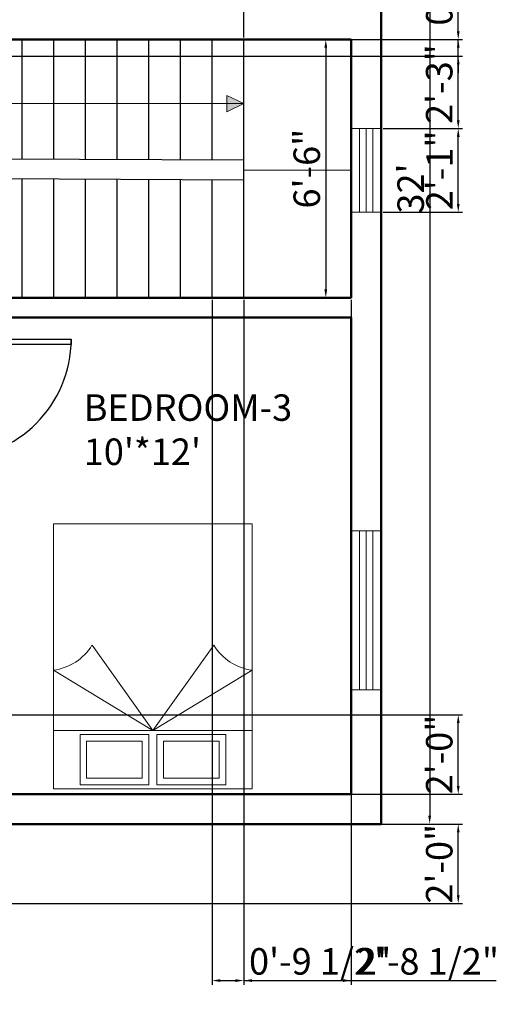
# Model space of a CAD drawing. Units: inches. Extents: x 2528 to 2954, y 1660 to 2209.
# Tile 3 of 4: x 2810 to 2954, y 1660 to 1957. Entities that reach past the tile are written whole.
import ezdxf

# ---------------------------------------------------------------- set-up
doc = ezdxf.new("R2010")
doc.units = ezdxf.units.IN
for name, color, linetype, lineweight in [('A-ANNO-DIMS', 5, 'Continuous', 18), ('A-ANNO-SYMB', 5, 'Continuous', 18), ('A-AREA-IDEN', 5, 'Continuous', 25), ('DOOR', 3, 'Continuous', 25), ('FURNITURE', 6, 'Continuous', 18), ('STEPS', 30, 'Continuous', 25), ('WALL', 1, 'Continuous', 50), ('WINDOW', 4, 'Continuous', 18)]:
    doc.layers.add(name, color=color, linetype=linetype, lineweight=lineweight)
doc.styles.get("Standard").update_dxf_attribs({"font": 'arial.ttf'})
doc.dimstyles.new('ISO-25', dxfattribs={"dimtxt": 8, "dimasz": 2.5, "dimexe": 1.25, "dimexo": 0.625, "dimtad": 1, "dimlunit": 3, "dimtxsty": 'Standard', "dimcen": 2.5, "dimadec": 0, "dimazin": 0, "dimtfac": 1, "dimtmove": 0, "dimatfit": 3, "dimfxl": 1, "dimarcsym": 0})

# ---------------------------------------------------------------- blocks, each defined once
blk = doc.blocks.new('*U2')
for p, q in [((0, 0), (0, -6)), ((40, 0), (40, -6))]:
    blk.add_line(p, q)
blk.add_lwpolyline([(0, 0), (0, 40), (1.75, 40), (1.75, 0)], close=True)
blk.add_arc((0, 0), 40, 0, 90)
blk = doc.blocks.new('*D12')
at = {"layer": 'A-ANNO-DIMS', "color": 0, "lineweight": -2, "transparency": 16777216}
for p, q in [((2919.54, 2098.39), (2934.84, 2098.39)), ((2933.59, 2095.89), (2933.59, 1716.89)), ((2919.54, 1714.39), (2934.84, 1714.39))]:
    blk.add_line(p, q, dxfattribs=at)
at = {"layer": 'A-ANNO-DIMS', "color": 0, "transparency": 16777216}
for points in [[(2933.17, 2095.89), (2934.01, 2095.89), (2933.59, 2098.39)], [(2933.17, 1716.89), (2934.01, 1716.89), (2933.59, 1714.39)]]:
    blk.add_solid(points, dxfattribs=at)
at = {"layer": 'Defpoints', "color": 0, "transparency": 16777216}
for p in [(2918.92, 2098.39), (2918.92, 1714.39), (2933.59, 1714.39)]:
    blk.add_point(p, dxfattribs=at)
at = {"layer": 'A-ANNO-DIMS', "color": 0, "transparency": 16777216, "insert": (2928.88, 1906.39), "char_height": 8, "attachment_point": 5, "rotation": 90}
blk.add_mtext("32'", dxfattribs=at)
blk = doc.blocks.new('*D13')
at = {"layer": 'A-ANNO-DIMS', "color": 0, "lineweight": -2, "transparency": 16777216}
for p, q in [((2878.05, 1951.39), (2903.46, 1951.39)), ((2902.21, 1948.89), (2902.21, 1875.89)), ((2878.05, 1873.39), (2903.46, 1873.39))]:
    blk.add_line(p, q, dxfattribs=at)
at = {"layer": 'A-ANNO-DIMS', "color": 0, "transparency": 16777216}
for points in [[(2901.79, 1948.89), (2902.63, 1948.89), (2902.21, 1951.39)], [(2901.79, 1875.89), (2902.63, 1875.89), (2902.21, 1873.39)]]:
    blk.add_solid(points, dxfattribs=at)
at = {"layer": 'Defpoints', "color": 0, "transparency": 16777216}
for p in [(2877.42, 1951.39), (2877.42, 1873.39), (2902.21, 1873.39)]:
    blk.add_point(p, dxfattribs=at)
at = {"layer": 'A-ANNO-DIMS', "color": 0, "transparency": 16777216, "insert": (2897.5, 1912.39), "char_height": 8, "attachment_point": 5, "rotation": 90}
blk.add_mtext('6\'-6"', dxfattribs=at)
blk = doc.blocks.new('BED-QUEEN-60X80')
for p, q in [((0, 0), (0, 80)), ((0, 80), (60, 80)), ((8, 78.8), (28.8, 78.8)), ((8, 65.6), (8, 78.8)), ((28.8, 78.8), (28.8, 63.6)), ((31.2, 78.8), (52, 78.8)), ((31.2, 65.6), (31.2, 78.8)), ((52, 78.8), (52, 63.6)), ((60, 80), (60, 0)), ((10, 76.8), (26.8, 76.8)), ((10, 65.6), (10, 76.8)), ((26.8, 76.8), (26.8, 65.6)), ((33.2, 65.6), (33.2, 76.8)), ((33.2, 76.8), (50, 76.8)), ((50, 76.8), (50, 65.6)), ((8, 63.6), (8, 65.6)), ((26.8, 65.6), (10, 65.6)), ((31.2, 63.6), (31.2, 65.6)), ((50, 65.6), (33.2, 65.6)), ((28.8, 63.6), (8, 63.6)), ((52, 63.6), (31.2, 63.6)), ((60, 62.4), (0, 62.4)), ((30, 62.4), (0, 44.18)), ((11.62, 36.62), (30, 62.4)), ((30, 62.4), (60, 44.18)), ((48.38, 36.62), (30, 62.4)), ((52, 62.4), (31.2, 62.4)), ((60, 0), (0, 0))]:
    blk.add_line(p, q)
for centre, start, end in [((-2.1, 28.24), 31.4416, 82.4986), ((62.1, 28.24), 97.5014, 148.5584)]:
    blk.add_arc(centre, 16.08, start, end)
blk = doc.blocks.new('WIN-48IN')
for p, q in [((0, 48), (9, 48)), ((2.5, 0), (2.5, 48)), ((4.5, 0), (4.5, 48)), ((6.5, 0), (6.5, 48)), ((9, 0), (0, 0))]:
    blk.add_line(p, q)
blk = doc.blocks.new('*D32')
at = {"layer": 'A-ANNO-DIMS', "color": 0, "lineweight": -2, "transparency": 16777216}
for p, q in [((2910.54, 1951.39), (2943.47, 1951.39)), ((2942.22, 1926.99), (2942.22, 1948.89)), ((2919.54, 1924.49), (2943.47, 1924.49))]:
    blk.add_line(p, q, dxfattribs=at)
at = {"layer": 'A-ANNO-DIMS', "color": 0, "transparency": 16777216}
for points in [[(2941.8, 1948.89), (2942.63, 1948.89), (2942.22, 1951.39)], [(2941.8, 1926.99), (2942.63, 1926.99), (2942.22, 1924.49)]]:
    blk.add_solid(points, dxfattribs=at)
at = {"layer": 'Defpoints', "color": 0, "transparency": 16777216}
for p in [(2909.92, 1951.39), (2942.22, 1951.39), (2918.92, 1924.49)]:
    blk.add_point(p, dxfattribs=at)
at = {"layer": 'A-ANNO-DIMS', "color": 0, "transparency": 16777216, "insert": (2937.5, 1937.94), "char_height": 8, "attachment_point": 5, "rotation": 90}
blk.add_mtext('2\'-3"', dxfattribs=at)
blk = doc.blocks.new('*D33')
at = {"layer": 'A-ANNO-DIMS', "color": 0, "lineweight": -2, "transparency": 16777216}
for p, q in [((2919.54, 1924.49), (2943.47, 1924.49)), ((2942.22, 1901.75), (2942.22, 1921.99)), ((2919.54, 1899.25), (2943.47, 1899.25))]:
    blk.add_line(p, q, dxfattribs=at)
at = {"layer": 'A-ANNO-DIMS', "color": 0, "transparency": 16777216}
for points in [[(2941.8, 1921.99), (2942.63, 1921.99), (2942.22, 1924.49)], [(2941.8, 1901.75), (2942.63, 1901.75), (2942.22, 1899.25)]]:
    blk.add_solid(points, dxfattribs=at)
at = {"layer": 'Defpoints', "color": 0, "transparency": 16777216}
for p in [(2918.92, 1924.49), (2942.22, 1924.49), (2918.92, 1899.25)]:
    blk.add_point(p, dxfattribs=at)
at = {"layer": 'A-ANNO-DIMS', "color": 0, "transparency": 16777216, "insert": (2937.57, 1911.87), "char_height": 8, "attachment_point": 5, "rotation": 90}
blk.add_mtext('2\'-1"', dxfattribs=at)
blk = doc.blocks.new('*D36')
at = {"layer": 'A-ANNO-DIMS', "color": 0, "lineweight": -2, "transparency": 16777216}
for p, q in [((2790.54, 1714.39), (2943.47, 1714.39)), ((2942.22, 1692.89), (2942.22, 1711.89)), ((2790.54, 1690.39), (2943.47, 1690.39))]:
    blk.add_line(p, q, dxfattribs=at)
at = {"layer": 'A-ANNO-DIMS', "color": 0, "transparency": 16777216}
for points in [[(2941.8, 1711.89), (2942.63, 1711.89), (2942.22, 1714.39)], [(2941.8, 1692.89), (2942.63, 1692.89), (2942.22, 1690.39)]]:
    blk.add_solid(points, dxfattribs=at)
at = {"layer": 'Defpoints', "color": 0, "transparency": 16777216}
for p in [(2789.92, 1714.39), (2942.22, 1714.39), (2789.92, 1690.39)]:
    blk.add_point(p, dxfattribs=at)
at = {"layer": 'A-ANNO-DIMS', "color": 0, "transparency": 16777216, "insert": (2937.51, 1702.39), "char_height": 8, "attachment_point": 5, "rotation": 90}
blk.add_mtext('2\'-0"', dxfattribs=at)
blk = doc.blocks.new('*D40')
at = {"layer": 'A-ANNO-DIMS', "color": 0, "lineweight": -2, "transparency": 16777216}
for p, q in [((2877.42, 1872.76), (2877.42, 1665.84)), ((2909.92, 1872.76), (2909.92, 1665.84)), ((2879.92, 1667.09), (2907.42, 1667.09)), ((2909.92, 1667.09), (2953.71, 1667.09))]:
    blk.add_line(p, q, dxfattribs=at)
at = {"layer": 'A-ANNO-DIMS', "color": 0, "transparency": 16777216}
for points in [[(2879.92, 1667.51), (2879.92, 1666.67), (2877.42, 1667.09)], [(2907.42, 1667.51), (2907.42, 1666.67), (2909.92, 1667.09)]]:
    blk.add_solid(points, dxfattribs=at)
at = {"layer": 'Defpoints', "color": 0, "transparency": 16777216}
for p in [(2877.42, 1873.39), (2909.92, 1873.39), (2909.92, 1667.09)]:
    blk.add_point(p, dxfattribs=at)
at = {"layer": 'A-ANNO-DIMS', "color": 0, "transparency": 16777216, "insert": (2933.06, 1671.85), "char_height": 8, "attachment_point": 5}
blk.add_mtext('2\'-8 1/2"', dxfattribs=at)
blk = doc.blocks.new('*D41')
at = {"layer": 'A-ANNO-DIMS', "color": 0, "lineweight": -2, "transparency": 16777216}
for p, q in [((2800.92, 1952.01), (2800.92, 2122.94)), ((2803.42, 2121.69), (2874.92, 2121.69)), ((2877.42, 1952.01), (2877.42, 2122.94))]:
    blk.add_line(p, q, dxfattribs=at)
at = {"layer": 'A-ANNO-DIMS', "color": 0, "transparency": 16777216}
for points in [[(2803.42, 2122.11), (2803.42, 2121.27), (2800.92, 2121.69)], [(2874.92, 2122.11), (2874.92, 2121.27), (2877.42, 2121.69)]]:
    blk.add_solid(points, dxfattribs=at)
at = {"layer": 'Defpoints', "color": 0, "transparency": 16777216}
for p in [(2877.42, 2121.69), (2800.92, 1951.39), (2877.42, 1951.39)]:
    blk.add_point(p, dxfattribs=at)
at = {"layer": 'A-ANNO-DIMS', "color": 0, "transparency": 16777216, "insert": (2839.17, 2126.45), "char_height": 8, "attachment_point": 5}
blk.add_mtext('6\'-4 1/2"', dxfattribs=at)
blk = doc.blocks.new('*D43')
at = {"layer": 'A-ANNO-DIMS', "color": 0, "lineweight": -2, "transparency": 16777216}
for p, q in [((2867.86, 1872.76), (2867.86, 1665.84)), ((2877.42, 1872.76), (2877.42, 1665.84)), ((2870.36, 1667.09), (2874.92, 1667.09)), ((2877.42, 1667.09), (2921.08, 1667.09))]:
    blk.add_line(p, q, dxfattribs=at)
at = {"layer": 'A-ANNO-DIMS', "color": 0, "transparency": 16777216}
for points in [[(2870.36, 1667.51), (2870.36, 1666.67), (2867.86, 1667.09)], [(2874.92, 1667.51), (2874.92, 1666.67), (2877.42, 1667.09)]]:
    blk.add_solid(points, dxfattribs=at)
at = {"layer": 'Defpoints', "color": 0, "transparency": 16777216}
for p in [(2867.86, 1873.39), (2877.42, 1873.39), (2877.42, 1667.09)]:
    blk.add_point(p, dxfattribs=at)
at = {"layer": 'A-ANNO-DIMS', "color": 0, "transparency": 16777216, "insert": (2900.5, 1671.85), "char_height": 8, "attachment_point": 5}
blk.add_mtext('0\'-9 1/2"', dxfattribs=at)
blk = doc.blocks.new('*D44')
at = {"layer": 'A-ANNO-DIMS', "color": 0, "lineweight": -2, "transparency": 16777216}
for p, q in [((2727.54, 1747.39), (2943.47, 1747.39)), ((2942.22, 1725.89), (2942.22, 1744.89)), ((2727.54, 1723.39), (2943.47, 1723.39))]:
    blk.add_line(p, q, dxfattribs=at)
at = {"layer": 'A-ANNO-DIMS', "color": 0, "transparency": 16777216}
for points in [[(2941.8, 1744.89), (2942.63, 1744.89), (2942.22, 1747.39)], [(2941.8, 1725.89), (2942.63, 1725.89), (2942.22, 1723.39)]]:
    blk.add_solid(points, dxfattribs=at)
at = {"layer": 'Defpoints', "color": 0, "transparency": 16777216}
for p in [(2726.92, 1747.39), (2942.22, 1747.39), (2726.92, 1723.39)]:
    blk.add_point(p, dxfattribs=at)
at = {"layer": 'A-ANNO-DIMS', "color": 0, "transparency": 16777216, "insert": (2937.51, 1735.39), "char_height": 8, "attachment_point": 5, "rotation": 90}
blk.add_mtext('2\'-0"', dxfattribs=at)
blk = doc.blocks.new('*D52')
at = {"layer": 'A-ANNO-DIMS', "color": 0, "lineweight": -2, "transparency": 16777216}
for p, q in [((2942.22, 1953.89), (2942.22, 1978.91)), ((2676.54, 1951.39), (2943.47, 1951.39)), ((2942.22, 1946.38), (2942.22, 1951.39)), ((2682.54, 1946.38), (2943.47, 1946.38)), ((2942.22, 1943.88), (2942.22, 1941.38))]:
    blk.add_line(p, q, dxfattribs=at)
at = {"layer": 'A-ANNO-DIMS', "color": 0, "transparency": 16777216}
for points in [[(2941.8, 1953.89), (2942.63, 1953.89), (2942.22, 1951.39)], [(2941.8, 1943.88), (2942.63, 1943.88), (2942.22, 1946.38)]]:
    blk.add_solid(points, dxfattribs=at)
at = {"layer": 'Defpoints', "color": 0, "transparency": 16777216}
for p in [(2675.92, 1951.39), (2942.22, 1951.39), (2681.92, 1946.38)]:
    blk.add_point(p, dxfattribs=at)
at = {"layer": 'A-ANNO-DIMS', "color": 0, "transparency": 16777216, "insert": (2937.51, 1967.65), "char_height": 8, "attachment_point": 5, "rotation": 90}
blk.add_mtext('0\'-5"', dxfattribs=at)

msp = doc.modelspace()

# ---------------------------------------------------------------- hatches: boundary and pattern name
at = {"layer": 'A-ANNO-SYMB'}
h = msp.add_hatch(color=256, dxfattribs=at)
h.dxf.hatch_style = 1
h.paths.add_polyline_path([(2872.336, 1934.474), (2872.336, 1932.092), (2877.423, 1932.092)])
h.paths.add_polyline_path([(2877.423, 1932.092), (2872.336, 1932.092), (2872.336, 1929.533)])

# ---------------------------------------------------------------- linework, layer by layer
for p, q in [((2872.336, 1929.533), (2872.336, 1934.474)), ((2872.336, 1934.474), (2877.423, 1932.092)), ((2787.908, 1932.092), (2877.423, 1932.092)), ((2877.423, 1932.092), (2872.336, 1929.533))]:
    msp.add_line(p, q, dxfattribs=at)
at = {"layer": 'STEPS'}
for p, q in [((2810.479, 1915.346), (2810.479, 1951.389)), ((2820.042, 1915.302), (2820.042, 1951.389)), ((2829.606, 1915.258), (2829.606, 1951.389)), ((2839.169, 1915.214), (2839.169, 1951.389)), ((2848.733, 1915.17), (2848.733, 1951.389)), ((2858.296, 1915.126), (2858.296, 1951.389)), ((2867.86, 1915.082), (2867.86, 1951.389)), ((2877.423, 1873.389), (2877.423, 1951.389)), ((2800.929, 1915.389), (2877.423, 1915.038)), ((2877.423, 1912.038), (2909.915, 1911.889)), ((2800.901, 1909.389), (2877.423, 1909.038)), ((2810.479, 1873.389), (2810.479, 1909.345)), ((2820.042, 1873.389), (2820.042, 1909.302)), ((2829.606, 1873.389), (2829.606, 1909.258)), ((2839.169, 1873.389), (2839.169, 1909.214)), ((2848.733, 1873.389), (2848.733, 1909.17)), ((2858.296, 1873.389), (2858.296, 1909.126)), ((2867.86, 1873.389), (2867.86, 1909.082))]:
    msp.add_line(p, q, dxfattribs=at)
at = {"layer": 'WALL'}
for p, q in [((2681.915, 1951.389), (2909.915, 1951.389)), ((2909.915, 1951.389), (2909.915, 1873.389)), ((2909.915, 1914.889), (2909.929, 1914.889)), ((2909.915, 1908.848), (2909.929, 1908.848)), ((2783.915, 1873.389), (2909.915, 1873.389)), ((2909.915, 1867.389), (2789.915, 1867.389)), ((2909.915, 1867.389), (2909.915, 1723.389)), ((2909.915, 1723.389), (2789.915, 1723.389))]:
    msp.add_line(p, q, dxfattribs=at)
msp.add_lwpolyline([(2618.915, 2098.389), (2918.915, 2098.389), (2918.915, 1714.389), (2618.915, 1714.389)], close=True, dxfattribs=at)
at = {"layer": 'WINDOW'}
for p, q in [((2909.915, 1924.491), (2918.915, 1924.491)), ((2912.415, 1924.491), (2912.415, 1911.869)), ((2914.415, 1924.491), (2914.415, 1911.869)), ((2916.415, 1924.491), (2916.415, 1911.869)), ((2912.415, 1899.246), (2912.415, 1911.869)), ((2914.415, 1899.246), (2914.415, 1911.869)), ((2916.415, 1899.246), (2916.415, 1911.869)), ((2909.915, 1899.246), (2918.915, 1899.246))]:
    msp.add_line(p, q, dxfattribs=at)

# ---------------------------------------------------------------- block references
at = {"layer": 'DOOR', "xscale": 0.9, "yscale": 0.9, "zscale": 0.9, "rotation": 270}
msp.add_blockref('*U2', (2789.315, 1860.866), dxfattribs=at)
at = {"layer": 'FURNITURE', "extrusion": (0, 0, -1), "zscale": -1, "rotation": 180}
msp.add_blockref('BED-QUEEN-60X80', (-2819.989, 1805.051), dxfattribs=at)
at = {"layer": 'WINDOW', "rotation": 180}
msp.add_blockref('WIN-48IN', (2918.915, 1802.925), dxfattribs=at)

# ---------------------------------------------------------------- texts
at = {"layer": 'A-AREA-IDEN', "insert": (2829.122, 1844.195), "char_height": 8, "attachment_point": 1}
msp.add_mtext_dynamic_manual_height_columns("BEDROOM-3\\P10'*12'", width=47.78448, gutter_width=12.5, heights=[0], dxfattribs=at)

# ---------------------------------------------------------------- dimensions: what is measured, and where the dimension line sits
at = {"layer": 'A-ANNO-DIMS'}
for base, p1, p2, picture, middle in [((2877.423, 2121.689), (2800.915, 1951.389), (2877.423, 1951.389), '*D41', (2839.169, 2126.451)), ((2877.423, 1667.089), (2867.86, 1873.389), (2877.423, 1873.389), '*D43', (2900.502, 1671.851)), ((2909.915, 1667.089), (2877.423, 1873.389), (2909.915, 1873.389), '*D40', (2933.062, 1671.851))]:
    dim = msp.add_linear_dim(base=base, p1=p1, p2=p2, dimstyle='ISO-25', override={"dimdec": 1, "dimlfac": 1, "dimrnd": 0, "dimzin": 1, "dimdsep": 46, "dimlunit": 4, "dimfrac": 2}, dxfattribs=at)
    dim.commit()
    dim.dimension.update_dxf_attribs({"geometry": picture, "text_midpoint": middle})
for base, p1, p2, override, picture, middle in [((2933.588, 1714.389), (2918.915, 2098.389), (2918.915, 1714.389), {"dimclrd": 0, "dimclre": 0, "dimclrt": 0}, '*D12', (2928.876, 1906.389)), ((2942.215, 1951.389), (2681.915, 1946.385), (2675.915, 1951.389), {"dimdec": 1, "dimlfac": 1, "dimrnd": 0, "dimzin": 1, "dimdsep": 46, "dimlunit": 4, "dimfrac": 2}, '*D52', (2937.505, 1967.647)), ((2902.209, 1873.389), (2877.423, 1951.389), (2877.423, 1873.389), {"dimclrd": 0, "dimclre": 0, "dimclrt": 0}, '*D13', (2897.499, 1912.389)), ((2942.215, 1951.389), (2918.915, 1924.491), (2909.915, 1951.389), {"dimdec": 1, "dimlfac": 1, "dimrnd": 0, "dimzin": 1, "dimdsep": 46, "dimlunit": 4, "dimfrac": 2}, '*D32', (2937.503, 1937.94)), ((2942.215, 1924.491), (2918.915, 1899.246), (2918.915, 1924.491), {"dimdec": 1, "dimlfac": 1, "dimrnd": 0, "dimzin": 1, "dimdsep": 46, "dimlunit": 4, "dimfrac": 2}, '*D33', (2937.574, 1911.869)), ((2942.215, 1747.389), (2726.915, 1723.389), (2726.915, 1747.389), {"dimdec": 1, "dimlfac": 1, "dimrnd": 0, "dimzin": 1, "dimdsep": 46, "dimlunit": 4, "dimfrac": 2}, '*D44', (2937.505, 1735.389)), ((2942.215, 1714.389), (2789.915, 1690.389), (2789.915, 1714.389), {"dimdec": 1, "dimlfac": 1, "dimrnd": 0, "dimzin": 1, "dimdsep": 46, "dimlunit": 4, "dimfrac": 2}, '*D36', (2937.505, 1702.389))]:
    dim = msp.add_linear_dim(base=base, p1=p1, p2=p2, angle=90, dimstyle='ISO-25', override=override, dxfattribs=at)
    dim.commit()
    dim.dimension.update_dxf_attribs({"geometry": picture, "text_midpoint": middle})

doc.saveas('drawing.dxf')
